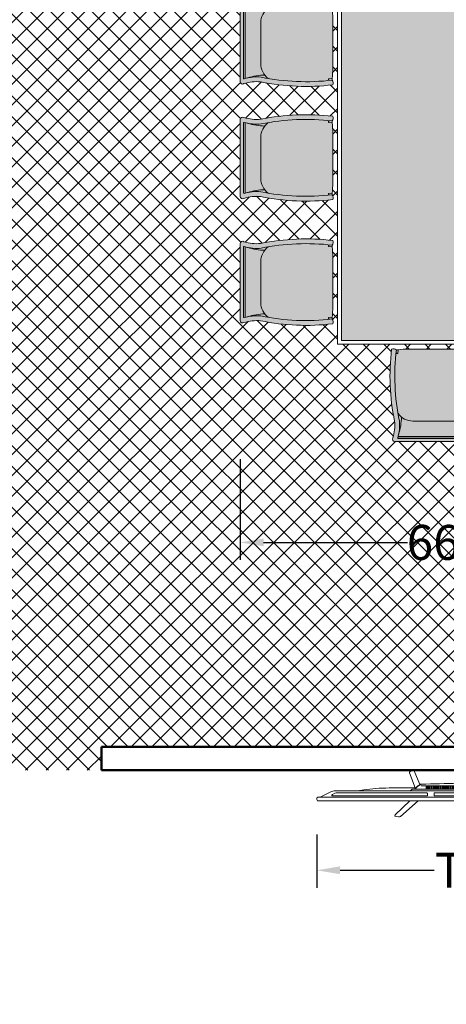
# Model space of a CAD drawing. Units: inches. Extents: x -466983 to 1020, y 324 to 318697.
# Tile 28 of 97: x 641 to 714, y 658 to 827. Entities that reach past the tile are written whole.
import ezdxf

# ---------------------------------------------------------------- set-up
doc = ezdxf.new("R2010")
doc.units = ezdxf.units.IN
doc.header["$MEASUREMENT"] = 0
for name, color, linetype, lineweight in [('A-ANNO-DIMS', 2, 'Continuous', 18), ('A-FLOR-PATT', 252, 'Continuous', 13), ('A-FURN', 8, 'Continuous', 18), ('A-WALL', 7, 'Continuous', 50)]:
    doc.layers.add(name, color=color, linetype=linetype, lineweight=lineweight)
doc.styles.get("Standard").update_dxf_attribs({"font": 'arial.ttf'})
doc.dimstyles.get("Standard").update_dxf_attribs({"dimtxt": 6, "dimasz": 4, "dimexe": 3, "dimexo": 3, "dimgap": 0.09, "dimtad": 0, "dimtih": 1, "dimtoh": 1, "dimdec": 1, "dimzin": 0, "dimdsep": 46, "dimlunit": 3, "dimtxsty": 'Standard', "dimcen": 0.09, "dimadec": 0, "dimazin": 0, "dimtfac": 1, "dimtdec": 1, "dimtofl": 0, "dimtmove": 0, "dimatfit": 3, "dimfxl": 1, "dimtolj": 1, "dimtzin": 0, "dimarcsym": 0})

# ---------------------------------------------------------------- blocks, each defined once
blk = doc.blocks.new('B2')
at = {"color": 0}
for points in [[(-161.1, -3.4), (-173.3, 26.2, 0.359324), (-175.3, 27.3, 0.097501), (-182.8, 24.2, 0.350578), (-183.5, 22.1), (-171.1, -10.4)], [(161.1, -3.4), (173.3, 26.2, -0.359324), (175.3, 27.3, -0.097501), (182.8, 24.2, -0.350578), (183.5, 22.1), (171.1, -10.4)], [(-381.9, -38.8, -0.13121), (-383.2, -32.7, -0.169032), (-383, -32.3), (-381.8, -31.1, -0.205713), (-381.3, -30.9), (-378.5, -30.9, 0.118206), (-376.2, -30.4), (-351.4, -18.4, -0.105648), (-345.8, -17), (0, -17)], [(-339.3, -21.2), (-339.3, -21.2, 0.099639), (-344.3, -22.2), (-349.2, -24.6, 0.215889), (-350.7, -26.3, 0.476075), (-349.4, -28, 0.244765)], [(-295.5, -17), (-282, -15, -0.02037), (-255.8, -12, -0.012056), (-227.2, -10.7), (-169.3, -10.7)], [(-181.8, -17), (-178.5, -14, -0.213415), (-177.3, -13.6), (0, -13.6)], [(-172.1, -13.6, -0.072098), (-159.2, -3, -0.121861), (-158.4, -2.8)], [(-170.1, -10.6, -0.053076), (-160.2, -2.9), (-158.4, -2.8)], [(-147.6, -13.6), (-147.6, -7.5, -0.414214), (-147.4, -7.3), (-146.5, -7.3, -0.414214), (-146.3, -7.5), (-146.3, -13.6)], [(-146.8, -28, 0.414214), (-145, -26.2), (-145, -23, 0.414214), (-146.8, -21.2)], [(-143.9, -13.6), (-143.9, -7.5, -0.414214), (-143.7, -7.3), (-142.7, -7.3, -0.414214), (-142.6, -7.5), (-142.6, -13.6)], [(-140.2, -13.6), (-140.2, -7.5, -0.414214), (-140, -7.3), (-139, -7.3, -0.414214), (-138.8, -7.5), (-138.8, -13.6)], [(-136.4, -13.6), (-136.4, -7.5, -0.414214), (-136.3, -7.3), (-135.3, -7.3, -0.414214), (-135.1, -7.5), (-135.1, -13.6)], [(-132.7, -13.6), (-132.7, -7.5, -0.414214), (-132.5, -7.3), (-131.6, -7.3, -0.414214), (-131.4, -7.5), (-131.4, -13.6)], [(-128.8, -28, -0.414214), (-130.6, -26.2), (-130.6, -23, -0.414214), (-128.8, -21.2)], [(-129, -13.6), (-129, -7.5, -0.414214), (-128.8, -7.3), (-127.9, -7.3, -0.414214), (-127.7, -7.5), (-127.7, -13.6)], [(-125.3, -13.6), (-125.3, -7.5, -0.414214), (-125.1, -7.3), (-124.1, -7.3, -0.414214), (-124, -7.5), (-124, -13.6)], [(-121.6, -13.6), (-121.6, -7.5, -0.414214), (-121.4, -7.3), (-120.4, -7.3, -0.414214), (-120.2, -7.5), (-120.2, -13.6)], [(-117.8, -13.6), (-117.8, -7.5, -0.414214), (-117.7, -7.3), (-116.7, -7.3, -0.414214), (-116.5, -7.5), (-116.5, -13.6)], [(-114.1, -13.6), (-114.1, -7.5, -0.414214), (-113.9, -7.3), (-113, -7.3, -0.414214), (-112.8, -7.5), (-112.8, -13.6)], [(-110.4, -13.6), (-110.4, -7.5, -0.414214), (-110.2, -7.3), (-109.3, -7.3, -0.414214), (-109.1, -7.5), (-109.1, -13.6)], [(-106.7, -13.6), (-106.7, -7.5, -0.414214), (-106.5, -7.3), (-105.5, -7.3, -0.414214), (-105.4, -7.5), (-105.4, -13.6)], [(-103, -13.6), (-103, -7.5, -0.414214), (-102.8, -7.3), (-101.8, -7.3, -0.414214), (-101.6, -7.5), (-101.6, -13.6)], [(-99.2, -13.6), (-99.2, -7.5, -0.414214), (-99.1, -7.3), (-98.1, -7.3, -0.414214), (-97.9, -7.5), (-97.9, -13.6)], [(-95.5, -13.6), (-95.5, -7.5, -0.414214), (-95.3, -7.3), (-94.4, -7.3, -0.414214), (-94.2, -7.5), (-94.2, -13.6)], [(-91.8, -13.6), (-91.8, -7.5, -0.414214), (-91.6, -7.3), (-90.7, -7.3, -0.414214), (-90.5, -7.5), (-90.5, -13.6)], [(-88.1, -13.6), (-88.1, -7.5, -0.414214), (-87.9, -7.3), (-86.9, -7.3, -0.414214), (-86.8, -7.5), (-86.8, -13.6)], [(-84.4, -13.6), (-84.4, -7.5, -0.414214), (-84.2, -7.3), (-83.2, -7.3, -0.414214), (-83, -7.5), (-83, -13.6)], [(-80.6, -13.6), (-80.6, -7.5, -0.414214), (-80.5, -7.3), (-79.5, -7.3, -0.414214), (-79.3, -7.5), (-79.3, -13.6)], [(-76.9, -13.6), (-76.9, -7.5, -0.414214), (-76.7, -7.3), (-75.8, -7.3, -0.414214), (-75.6, -7.5), (-75.6, -13.6)], [(-73.2, -13.6), (-73.2, -7.5, -0.414214), (-73, -7.3), (-72.1, -7.3, -0.414214), (-71.9, -7.5), (-71.9, -13.6)], [(-69.5, -13.6), (-69.5, -7.5, -0.414214), (-69.3, -7.3), (-68.3, -7.3, -0.414214), (-68.2, -7.5), (-68.2, -13.6)], [(-65.8, -13.6), (-65.8, -7.5, -0.414214), (-65.6, -7.3), (-64.6, -7.3, -0.414214), (-64.4, -7.5), (-64.4, -13.6)], [(-62, -13.6), (-62, -7.5, -0.414214), (-61.9, -7.3), (-60.9, -7.3, -0.414214), (-60.7, -7.5), (-60.7, -13.6)], [(-58.3, -13.6), (-58.3, -7.5, -0.414214), (-58.1, -7.3), (-57.2, -7.3, -0.414214), (-57, -7.5), (-57, -13.6)], [(-54.6, -13.6), (-54.6, -7.5, -0.414214), (-54.4, -7.3), (-53.5, -7.3, -0.414214), (-53.3, -7.5), (-53.3, -13.6)], [(-50.9, -13.6), (-50.9, -7.5, -0.414214), (-50.7, -7.3), (-49.7, -7.3, -0.414214), (-49.6, -7.5), (-49.6, -13.6)], [(-47.2, -13.6), (-47.2, -7.5, -0.414214), (-47, -7.3), (-46, -7.3, -0.414214), (-45.8, -7.5), (-45.8, -13.6)], [(-43.4, -13.6), (-43.4, -7.5, -0.414214), (-43.3, -7.3), (-42.3, -7.3, -0.414214), (-42.1, -7.5), (-42.1, -13.6)], [(-39.7, -13.6), (-39.7, -7.5, -0.414214), (-39.5, -7.3), (-38.6, -7.3, -0.414214), (-38.4, -7.5), (-38.4, -13.6)], [(-36, -13.6), (-36, -7.5, -0.414214), (-35.8, -7.3), (-34.9, -7.3, -0.414214), (-34.7, -7.5), (-34.7, -13.6)], [(-32.3, -13.6), (-32.3, -7.5, -0.414214), (-32.1, -7.3), (-31.1, -7.3, -0.414214), (-31, -7.5), (-31, -13.6)], [(-28.6, -13.6), (-28.6, -7.5, -0.414214), (-28.4, -7.3), (-27.4, -7.3, -0.414214), (-27.2, -7.5), (-27.2, -13.6)], [(-24.8, -13.6), (-24.8, -7.5, -0.414214), (-24.7, -7.3), (-23.7, -7.3, -0.414214), (-23.5, -7.5), (-23.5, -13.6)], [(-21.1, -13.6), (-21.1, -7.5, -0.414214), (-20.9, -7.3), (-20, -7.3, -0.414214), (-19.8, -7.5), (-19.8, -13.6)], [(-17.4, -13.6), (-17.4, -7.5, -0.414214), (-17.2, -7.3), (-16.3, -7.3, -0.414214), (-16.1, -7.5), (-16.1, -13.6)], [(-13.7, -13.6), (-13.7, -7.5, -0.414214), (-13.5, -7.3), (-12.5, -7.3, -0.414214), (-12.4, -7.5), (-12.4, -13.6)], [(-10, -13.6), (-10, -7.5, -0.414214), (-9.8, -7.3), (-8.8, -7.3, -0.414214), (-8.6, -7.5), (-8.6, -13.6)], [(-10, -28, 0.414214), (-8.2, -26.2), (-8.2, -23, 0.414214), (-10, -21.2)], [(-6.2, -13.6), (-6.2, -7.5, -0.414214), (-6.1, -7.3), (-5.1, -7.3, -0.414214), (-4.9, -7.5), (-4.9, -13.6)], [(-2.5, -13.6), (-2.5, -7.5, -0.414214), (-2.3, -7.3), (-1.4, -7.3, -0.414214), (-1.2, -7.5), (-1.2, -13.6)], [(181.8, -17), (178.5, -14, 0.213415), (177.3, -13.6), (0, -13.6)], [(381.9, -38.8, 0.13121), (383.2, -32.7, 0.169032), (383, -32.3), (381.8, -31.1, 0.205713), (381.3, -30.9), (378.5, -30.9, -0.118206), (376.2, -30.4), (351.4, -18.4, 0.105648), (345.8, -17), (0, -17)], [(2.5, -13.6), (2.5, -7.5, 0.414214), (2.3, -7.3), (1.4, -7.3, 0.414214), (1.2, -7.5), (1.2, -13.6)], [(6.2, -13.6), (6.2, -7.5, 0.414214), (6.1, -7.3), (5.1, -7.3, 0.414214), (4.9, -7.5), (4.9, -13.6)], [(10, -28, -0.414214), (8.2, -26.2), (8.2, -23, -0.414214), (10, -21.2)], [(10, -13.6), (10, -7.5, 0.414214), (9.8, -7.3), (8.8, -7.3, 0.414214), (8.6, -7.5), (8.6, -13.6)], [(13.7, -13.6), (13.7, -7.5, 0.414214), (13.5, -7.3), (12.5, -7.3, 0.414214), (12.4, -7.5), (12.4, -13.6)], [(17.4, -13.6), (17.4, -7.5, 0.414214), (17.2, -7.3), (16.3, -7.3, 0.414214), (16.1, -7.5), (16.1, -13.6)], [(21.1, -13.6), (21.1, -7.5, 0.414214), (20.9, -7.3), (20, -7.3, 0.414214), (19.8, -7.5), (19.8, -13.6)], [(24.8, -13.6), (24.8, -7.5, 0.414214), (24.7, -7.3), (23.7, -7.3, 0.414214), (23.5, -7.5), (23.5, -13.6)], [(28.6, -13.6), (28.6, -7.5, 0.414214), (28.4, -7.3), (27.4, -7.3, 0.414214), (27.2, -7.5), (27.2, -13.6)], [(32.3, -13.6), (32.3, -7.5, 0.414214), (32.1, -7.3), (31.1, -7.3, 0.414214), (31, -7.5), (31, -13.6)], [(36, -13.6), (36, -7.5, 0.414214), (35.8, -7.3), (34.9, -7.3, 0.414214), (34.7, -7.5), (34.7, -13.6)], [(39.7, -13.6), (39.7, -7.5, 0.414214), (39.5, -7.3), (38.6, -7.3, 0.414214), (38.4, -7.5), (38.4, -13.6)], [(43.4, -13.6), (43.4, -7.5, 0.414214), (43.3, -7.3), (42.3, -7.3, 0.414214), (42.1, -7.5), (42.1, -13.6)], [(47.2, -13.6), (47.2, -7.5, 0.414214), (47, -7.3), (46, -7.3, 0.414214), (45.8, -7.5), (45.8, -13.6)], [(50.9, -13.6), (50.9, -7.5, 0.414214), (50.7, -7.3), (49.7, -7.3, 0.414214), (49.6, -7.5), (49.6, -13.6)], [(54.6, -13.6), (54.6, -7.5, 0.414214), (54.4, -7.3), (53.5, -7.3, 0.414214), (53.3, -7.5), (53.3, -13.6)], [(58.3, -13.6), (58.3, -7.5, 0.414214), (58.1, -7.3), (57.2, -7.3, 0.414214), (57, -7.5), (57, -13.6)], [(62, -13.6), (62, -7.5, 0.414214), (61.9, -7.3), (60.9, -7.3, 0.414214), (60.7, -7.5), (60.7, -13.6)], [(65.8, -13.6), (65.8, -7.5, 0.414214), (65.6, -7.3), (64.6, -7.3, 0.414214), (64.4, -7.5), (64.4, -13.6)], [(69.5, -13.6), (69.5, -7.5, 0.414214), (69.3, -7.3), (68.3, -7.3, 0.414214), (68.2, -7.5), (68.2, -13.6)], [(73.2, -13.6), (73.2, -7.5, 0.414214), (73, -7.3), (72.1, -7.3, 0.414214), (71.9, -7.5), (71.9, -13.6)], [(76.9, -13.6), (76.9, -7.5, 0.414214), (76.7, -7.3), (75.8, -7.3, 0.414214), (75.6, -7.5), (75.6, -13.6)], [(80.6, -13.6), (80.6, -7.5, 0.414214), (80.5, -7.3), (79.5, -7.3, 0.414214), (79.3, -7.5), (79.3, -13.6)], [(84.4, -13.6), (84.4, -7.5, 0.414214), (84.2, -7.3), (83.2, -7.3, 0.414214), (83, -7.5), (83, -13.6)], [(88.1, -13.6), (88.1, -7.5, 0.414214), (87.9, -7.3), (86.9, -7.3, 0.414214), (86.8, -7.5), (86.8, -13.6)], [(91.8, -13.6), (91.8, -7.5, 0.414214), (91.6, -7.3), (90.7, -7.3, 0.414214), (90.5, -7.5), (90.5, -13.6)], [(95.5, -13.6), (95.5, -7.5, 0.414214), (95.3, -7.3), (94.4, -7.3, 0.414214), (94.2, -7.5), (94.2, -13.6)], [(99.2, -13.6), (99.2, -7.5, 0.414214), (99.1, -7.3), (98.1, -7.3, 0.414214), (97.9, -7.5), (97.9, -13.6)], [(103, -13.6), (103, -7.5, 0.414214), (102.8, -7.3), (101.8, -7.3, 0.414214), (101.6, -7.5), (101.6, -13.6)], [(106.7, -13.6), (106.7, -7.5, 0.414214), (106.5, -7.3), (105.5, -7.3, 0.414214), (105.4, -7.5), (105.4, -13.6)], [(110.4, -13.6), (110.4, -7.5, 0.414214), (110.2, -7.3), (109.3, -7.3, 0.414214), (109.1, -7.5), (109.1, -13.6)], [(114.1, -13.6), (114.1, -7.5, 0.414214), (113.9, -7.3), (113, -7.3, 0.414214), (112.8, -7.5), (112.8, -13.6)], [(117.8, -13.6), (117.8, -7.5, 0.414214), (117.7, -7.3), (116.7, -7.3, 0.414214), (116.5, -7.5), (116.5, -13.6)], [(121.6, -13.6), (121.6, -7.5, 0.414214), (121.4, -7.3), (120.4, -7.3, 0.414214), (120.2, -7.5), (120.2, -13.6)], [(125.3, -13.6), (125.3, -7.5, 0.414214), (125.1, -7.3), (124.1, -7.3, 0.414214), (124, -7.5), (124, -13.6)], [(129, -13.6), (129, -7.5, 0.414214), (128.8, -7.3), (127.9, -7.3, 0.414214), (127.7, -7.5), (127.7, -13.6)], [(128.8, -28, 0.414214), (130.6, -26.2), (130.6, -23, 0.414214), (128.8, -21.2)], [(132.7, -13.6), (132.7, -7.5, 0.414214), (132.5, -7.3), (131.6, -7.3, 0.414214), (131.4, -7.5), (131.4, -13.6)], [(136.4, -13.6), (136.4, -7.5, 0.414214), (136.3, -7.3), (135.3, -7.3, 0.414214), (135.1, -7.5), (135.1, -13.6)], [(140.2, -13.6), (140.2, -7.5, 0.414214), (140, -7.3), (139, -7.3, 0.414214), (138.8, -7.5), (138.8, -13.6)], [(143.9, -13.6), (143.9, -7.5, 0.414214), (143.7, -7.3), (142.7, -7.3, 0.414214), (142.6, -7.5), (142.6, -13.6)], [(146.8, -28, -0.414214), (145, -26.2), (145, -23, -0.414214), (146.8, -21.2)], [(147.6, -13.6), (147.6, -7.5, 0.414214), (147.4, -7.3), (146.5, -7.3, 0.414214), (146.3, -7.5), (146.3, -13.6)], [(172.1, -13.6, 0.072098), (159.2, -3, 0.121861), (158.4, -2.8)], [(170.1, -10.6, 0.053076), (160.2, -2.9), (158.4, -2.8)], [(295.5, -17), (282, -15, 0.02037), (255.8, -12, 0.012056), (227.2, -10.7), (169.3, -10.7)], [(339.3, -21.2), (339.3, -21.2, -0.099639), (344.3, -22.2), (349.2, -24.6, -0.215889), (350.7, -26.3, -0.476075), (349.4, -28, -0.244765)], [(-182.5, -38.8), (-214.4, -69.1, 0.250582), (-215, -71, 0.266718), (-214.3, -71.9, 0.084688)], [(-214.3, -71.9), (-207.3, -73.1, 0.211205), (-203.3, -72.1), (-165.2, -38.8)], [(214.3, -71.9), (207.3, -73.1, -0.211205), (203.3, -72.1), (165.2, -38.8)], [(182.5, -38.8), (214.4, -69.1, -0.250582), (215, -71, -0.266718), (214.3, -71.9, -0.084688)]]:
    blk.add_lwpolyline(points, format="xyb", dxfattribs=at)
for points in [[(-339.3, -21.2), (-146.8, -21.2)], [(-158.6, -6.5), (0, -6.5)], [(-128.8, -21.2), (-10, -21.2)], [(158.6, -6.5), (0, -6.5)], [(128.8, -21.2), (10, -21.2)], [(339.3, -21.2), (146.8, -21.2)], [(-381.9, -38.8), (0, -38.8)], [(-378.5, -30.9), (0, -30.9)], [(-349.4, -28), (-146.8, -28)], [(-128.8, -28), (-10, -28)], [(378.5, -30.9), (0, -30.9)], [(381.9, -38.8), (0, -38.8)], [(128.8, -28), (10, -28)], [(349.4, -28), (146.8, -28)]]:
    blk.add_lwpolyline(points, dxfattribs=at)
for centre, radius, start, end in [((0, -4564), 4564, 90, 91.9893), ((0, -4564), 4564, 88.0107, 90), ((-170.5, -10.1), 0.6, 200.9784, 314.0295), ((170.5, -10.1), 0.6, 225.9705, 339.0216)]:
    blk.add_arc(centre, radius, start, end, dxfattribs=at)
blk = doc.blocks.new('A$C51F1')
h = blk.add_hatch(color=256)
h.dxf.hatch_style = 1
h.paths.add_polyline_path([(0.4279, 0.4929), (0.026, 0.4929, 0.585109), (0.0153, 0.4737, -0.102523), (0.0249, 0.3863, 0.080461), (0.0093, 0.0091, 0.3023), (0.0338, 0.012, -0.012942), (0.0343, 0.0123, -0.080591), (0.05, 0.3835, 0.086627), (0.0435, 0.4661, -0.308377), (0.0433, 0.4665, -0.237278), (0.0433, 0.4671, 0.005839), (0.0418, 0.4726, -0.471786), (0.0436, 0.4758), (0.2273, 0.4758), (0.4111, 0.4758, -0.471786), (0.4129, 0.4726, 0.005839), (0.4114, 0.4671, -0.293853), (0.4112, 0.4664, 0.08699), (0.4047, 0.3835, -0.080655), (0.4203, 0.012, 0.301773), (0.4447, 0.0091, 0.080461), (0.4291, 0.3863, -0.102523), (0.4387, 0.4737, 0.587111)])
h.paths.add_polyline_path([(0.4107, 0.4676), (0.2273, 0.4676), (0.0439, 0.4676, 0.311255), (0.0433, 0.4671, -0.000568), (0.0434, 0.4666, -0.365297), (0.0439, 0.4668), (0.2273, 0.4668), (0.4107, 0.4668, -0.365297), (0.4113, 0.4666, -0.000568), (0.4114, 0.4671, 0.311255)], flags=17)
h = blk.add_hatch(color=256)
h.dxf.hatch_style = 1
h.paths.add_polyline_path([(0.4117, 0.3464, 0.23459), (0.3341, 0.3858), (0.2273, 0.3858), (0.1205, 0.3858, 0.165743), (0.061, 0.3649, 0.071703), (0.0463, 0.4542, -0.071168), (0.0502, 0.3861, 0.080361), (0.0343, 0.0123, -0.184513), (0.0429, 0.0127, 0.028193), (0.097, 0.0091), (0.227, 0.0091), (0.3571, 0.0091, 0.028193), (0.4111, 0.0127, -0.198751), (0.4203, 0.012, 0.072468)])
h.paths.add_polyline_path([(0.4084, 0.4542, -0.01323), (0.4113, 0.4666, 0.365297), (0.4107, 0.4668, 0.310553), (0.4107, 0.4676), (0.0439, 0.4676, 0.311255), (0.0433, 0.4671, -0.013798), (0.0463, 0.4542, -0.071703), (0.061, 0.3649, -0.165743), (0.1205, 0.3858), (0.2273, 0.3858), (0.3341, 0.3858, -0.165743), (0.3937, 0.3649, -0.071703)])
h.paths.add_polyline_path([(0.4047, 0.3835, -0.073923), (0.4084, 0.4542, 0.071703), (0.3937, 0.3649, -0.06627), (0.4117, 0.3464, 0.008137)], flags=17)
h.paths.add_polyline_path([(0.413, 0.473, 0.415817), (0.4111, 0.4758), (0.0436, 0.4758, 0.415817), (0.0416, 0.473, -0.006308), (0.0433, 0.4671, -0.311255), (0.0439, 0.4676), (0.4107, 0.4676, -0.336555), (0.4114, 0.4671, -0.006308)])
h = blk.add_hatch(color=256)
h.dxf.hatch_style = 1
h.paths.add_polyline_path([(0.4084, 0.4542, -0.01323), (0.4113, 0.4666, 0.365297), (0.4107, 0.4668), (0.2273, 0.4668), (0.0436, 0.4668, 0.193526), (0.0434, 0.4666, -0.01323), (0.0463, 0.4542, -0.071703), (0.061, 0.3649, -0.165743), (0.1205, 0.3858), (0.2273, 0.3858), (0.3341, 0.3858, -0.165743), (0.3937, 0.3649, -0.071703)])
at = {"color": 0}
for p, q in [((0.0436, 0.4758), (0.4111, 0.4758)), ((0.0439, 0.4676), (0.4107, 0.4676)), ((0.2273, 0.4668), (0.0439, 0.4668)), ((0.2273, 0.4668), (0.4107, 0.4668)), ((0.2273, 0.3858), (0.1205, 0.3858)), ((0.2273, 0.3858), (0.3341, 0.3858)), ((0.0417, 0.0321), (0.0321, 0.0321)), ((0.0417, 0.0321), (0.0326, 0.0278)), ((0.0435, 0.0127), (0.0417, 0.0321)), ((0.4112, 0.0127), (0.4129, 0.0321)), ((0.4129, 0.0321), (0.4225, 0.0321)), ((0.4129, 0.0321), (0.4221, 0.0278))]:
    blk.add_line(p, q, dxfattribs=at)
blk.add_lwpolyline([(0.4387, 0.4737, 0.102523), (0.4291, 0.3863, -0.080461), (0.4447, 0.0091, -0.3023), (0.4203, 0.012, 0.197932), (0.4111, 0.0127, -0.028193), (0.3571, 0.0091), (0.227, 0.0091), (0.097, 0.0091, -0.028193), (0.0429, 0.0127, 0.197932), (0.0338, 0.012, -0.3023), (0.0093, 0.0091, -0.080461), (0.0249, 0.3863, 0.102523), (0.0153, 0.4737, -0.587111), (0.0261, 0.4929), (0.4279, 0.4929, -0.587111)], format="xyb", close=True, dxfattribs=at)
for centre, radius, start, end in [((0.044, 0.4735), 0.00242, 100.345, 201.3742), ((-0.1898, 0.4063), 0.2409, 355.1793, 16.07), ((0.0439, 0.4669), 0.000725, 87.3762, 197.5208), ((0.0438, 0.4664), 0.000433, 71.7715, 189.2202), ((0.6445, 0.4063), 0.2409, 164.0374, 185.4487), ((0.4107, 0.4669), 0.000725, 342.4792, 92.6238), ((0.4109, 0.4664), 0.000433, 350.7798, 108.2285), ((0.4106, 0.4735), 0.00242, 338.6258, 79.655), ((-0.2563, 0.3584), 0.3173, 1.1591, 17.5641), ((0.7109, 0.3584), 0.3173, 162.4359, 178.8409), ((1.1976, 0.1501), 1.1714, 168.378, 186.769), ((0.1214, 0.2879), 0.0978, 90.5164, 143.1927), ((0.3332, 0.2879), 0.0978, 36.8073, 89.4836), ((-0.7314, 0.1497), 1.1599, 353.1854, 11.6291), ((0.0397, 0.0013), 0.012, 71.7536, 116.5375), ((0.4149, 0.0013), 0.012, 63.4625, 108.2464)]:
    blk.add_arc(centre, radius, start, end, dxfattribs=at)
blk = doc.blocks.new('Dining Table 1')
h = blk.add_hatch(color=256)
h.dxf.hatch_style = 1
h.set_gradient(color1=(0, 107, 0), color2=(254, 234, 185), name='INVSPHERICAL')
h.paths.add_polyline_path([(1939.98, 1142.68), (1908.44, 1142.68), (1908.44, 1061.84), (1939.98, 1061.84)])
at = {"ltscale": 0.5}
for points in [[(1907.78, 1143.33), (1907.78, 1061.19), (1940.64, 1061.19), (1940.64, 1143.33)], [(1908.44, 1142.68), (1908.44, 1061.84), (1939.98, 1061.84), (1939.98, 1142.68)]]:
    blk.add_lwpolyline(points, close=True, dxfattribs=at)
at = {"ltscale": 0.5, "xscale": 32.85880592291654, "yscale": 32.85880592291654, "zscale": 32.85880592291654}
blk.add_blockref('A$C51F1', (1916.75, 1143.86), dxfattribs=at)
at = {"ltscale": 0.5, "yscale": 32.85880592291654, "zscale": 32.85880592291654}
for p, xscale, rotation in [((1907.26, 1140.11), -32.85880592291654, 90), ((1941.16, 1140.11), 32.85880592291654, 270), ((1907.26, 1120.4), -32.85880592291654, 90), ((1941.16, 1120.4), 32.85880592291654, 270), ((1907.26, 1085.76), 32.85880592291654, 89.99999999999999), ((1941.16, 1085.76), -32.85880592291654, 270), ((1907.26, 1064.41), 32.85880592291654, 89.99999999999999), ((1941.16, 1064.41), -32.85880592291654, 270), ((1916.75, 1060.66), -32.85880592291654, 180)]:
    blk.add_blockref('A$C51F1', p, dxfattribs=dict(at, xscale=xscale, rotation=rotation))
blk = doc.blocks.new('*D101')
at = {"layer": 'A-ANNO-DIMS', "color": 0, "lineweight": -2, "transparency": 16777216}
for p, q in [((691.81, 686.91), (691.81, 677.75)), ((752.9, 686.91), (752.9, 677.75)), ((695.81, 680.75), (711.95, 680.75)), ((748.9, 680.75), (732.76, 680.75))]:
    blk.add_line(p, q, dxfattribs=at)
at = {"layer": 'A-ANNO-DIMS', "color": 0, "transparency": 16777216}
for points in [[(695.81, 681.42), (695.81, 680.08), (691.81, 680.75)], [(748.9, 681.42), (748.9, 680.08), (752.9, 680.75)]]:
    blk.add_solid(points, dxfattribs=at)
at = {"layer": 'Defpoints', "color": 0, "transparency": 16777216}
for p in [(691.81, 689.91), (752.9, 689.91), (752.9, 680.75)]:
    blk.add_point(p, dxfattribs=at)
at = {"layer": 'A-ANNO-DIMS', "color": 0, "transparency": 16777216, "insert": (722.35, 680.75), "char_height": 6, "attachment_point": 5}
blk.add_mtext('\\A1;TV 61', dxfattribs=at)
blk = doc.blocks.new('*D112')
at = {"layer": 'A-ANNO-DIMS', "color": 0, "lineweight": -2, "transparency": 16777216}
for p, q in [((678.65, 751.43), (678.65, 734.1)), ((744.94, 751.43), (744.94, 734.1)), ((682.65, 737.1), (707.39, 737.1)), ((740.94, 737.1), (716.2, 737.1))]:
    blk.add_line(p, q, dxfattribs=at)
at = {"layer": 'A-ANNO-DIMS', "color": 0, "transparency": 16777216}
for points in [[(682.65, 737.76), (682.65, 736.43), (678.65, 737.1)], [(740.94, 737.76), (740.94, 736.43), (744.94, 737.1)]]:
    blk.add_solid(points, dxfattribs=at)
at = {"layer": 'Defpoints', "color": 0, "transparency": 16777216}
for p in [(678.65, 754.43), (744.94, 754.43), (744.94, 737.1)]:
    blk.add_point(p, dxfattribs=at)
at = {"layer": 'A-ANNO-DIMS', "color": 0, "transparency": 16777216, "insert": (711.79, 737.1), "char_height": 6, "attachment_point": 5}
blk.add_mtext('\\A1;66', dxfattribs=at)

msp = doc.modelspace()

# ---------------------------------------------------------------- hatches: boundary and pattern name
at = {"layer": 'A-FLOR-PATT', "transparency": 33554572}
h = msp.add_hatch(dxfattribs=at)
h.set_pattern_fill('ANSI37', color=256, scale=30)
h.set_pattern_definition([(45, (-1212.4137, -290.035), (-2.6516504, 2.6516504), []), (135, (-1212.4137, -290.035), (-2.6516504, -2.6516504), [])])
h.paths.add_polyline_path([(901.81, 1075.94), (900.61, 1075.94), (900.61, 1065.39), (899.39, 1065.39), (898.09, 1065.39), (892.84, 1058.71, -0.258377), (892.19, 1058.35), (879.98, 1058.35, -0.20177), (879.44, 1058.58), (874.08, 1065.39), (872.78, 1065.39), (871.56, 1065.39), (871.56, 1075.94), (813.81, 1075.94), (813.81, 1044.79), (832.39, 1044.79, -0.394795), (848.66, 1028.54), (848.66, 1009.94), (901.81, 1009.94), (901.81, 1015.94), (901.31, 1015.94), (871.31, 1015.94), (871.31, 1017.25), (871.33, 1017.25, -0.401453), (901.31, 1045.94), (901.81, 1045.94)])
edge = h.paths.add_edge_path(flags=16)
edge.add_line((847.77, 1068.95), (847.77, 1073.71))
edge.add_arc((849.23, 1073.71), 1.45, 90, 180, ccw=False)
edge.add_line((849.23, 1075.16), (864.49, 1075.16))
edge.add_arc((864.49, 1073.71), 1.45, 0, 90, ccw=False)
edge.add_line((865.95, 1073.71), (865.95, 1069))
edge.add_arc((832.64, 1068.98), 33.3, -20.6123, 0.0472, ccw=False)
edge.add_ellipse((856.86, 1058.48), major_axis=(0, 10.21), ratio=0.685919, start_angle=100.0088, end_angle=259.9912, ccw=False)
edge.add_arc((881.07, 1068.98), 33.3, 180.0472, 200.6123, ccw=False)
h.paths.add_polyline_path([(853.15, 1066.48), (853.15, 1066.45), (853.15, 1066.45, 0.433107), (852.92, 1066.68), (852.92, 1066.45), (853.15, 1066.45), (853.15, 1066.48), (853.09, 1066.61, 0.697939), (852.7, 1066.45), (852.7, 1066.45), (852.7, 1066.48), (852.92, 1067), (852.92, 1066.68, -0.396254)], flags=0)
h.paths.add_polyline_path([(861.02, 1066.48), (861.02, 1066.45), (861.02, 1066.45, 0.416404), (860.8, 1066.68), (860.8, 1066.45), (861.02, 1066.45), (861.02, 1066.48), (860.97, 1066.61, 0.713344), (860.57, 1066.45), (860.57, 1066.45), (860.57, 1066.48), (860.8, 1067), (860.8, 1066.68, -0.379973)], flags=0)
edge = h.paths.add_edge_path(flags=0)
edge.add_spline(control_points=[(861.13, 1065.79), (861.47, 1065.25), (861.61, 1065.02), (861.98, 1064.37), (862.19, 1063.94), (862.56, 1063.04), (862.72, 1062.56), (862.99, 1061.58), (863.09, 1061.07), (863.25, 1060.03), (863.29, 1059.5), (863.33, 1058.44), (863.32, 1057.91), (863.24, 1056.85), (863.17, 1056.33), (862.97, 1055.31), (862.84, 1054.81), (862.54, 1053.85), (862.36, 1053.39), (861.95, 1052.52), (861.73, 1052.12), (861.23, 1051.36), (860.97, 1051.02), (860.4, 1050.39), (860.11, 1050.12), (859.49, 1049.65), (859.18, 1049.45), (858.53, 1049.13), (858.2, 1049.01), (857.53, 1048.85), (857.2, 1048.81), (856.52, 1048.81), (856.19, 1048.85), (855.52, 1049.01), (855.19, 1049.13), (854.54, 1049.45), (854.23, 1049.64), (853.61, 1050.12), (853.32, 1050.39), (852.75, 1051.01), (852.49, 1051.36), (852, 1052.11), (851.77, 1052.52), (851.36, 1053.39), (851.18, 1053.85), (850.88, 1054.81), (850.75, 1055.31), (850.55, 1056.33), (850.48, 1056.85), (850.4, 1057.9), (850.39, 1058.44), (850.43, 1059.5), (850.47, 1060.03), (850.63, 1061.07), (850.73, 1061.58), (851, 1062.56), (851.16, 1063.04), (851.53, 1063.94), (851.73, 1064.37), (852.11, 1065.02), (852.25, 1065.25), (852.61, 1065.73)], knot_values=[3.915332, 3.915332, 3.915332, 3.915332, 4.013468, 4.013468, 4.175532, 4.175532, 4.337596, 4.337596, 4.49966, 4.49966, 4.661724, 4.661724, 4.823788, 4.823788, 4.985852, 4.985852, 5.147916, 5.147916, 5.30998, 5.30998, 5.472044, 5.472044, 5.634109, 5.634109, 5.796173, 5.796173, 5.958237, 5.958237, 6.120301, 6.120301, 6.282365, 6.282365, 6.444429, 6.444429, 6.606493, 6.606493, 6.768557, 6.768557, 6.930621, 6.930621, 7.092685, 7.092685, 7.254749, 7.254749, 7.416813, 7.416813, 7.578878, 7.578878, 7.740942, 7.740942, 7.903006, 7.903006, 8.06507, 8.06507, 8.227134, 8.227134, 8.389198, 8.389198, 8.551262, 8.551262, 8.65037, 8.65037, 8.65037, 8.65037], degree=3, periodic=0)
edge.add_line((852.64, 1065.79), (861.13, 1065.79))
edge = h.paths.add_edge_path(flags=0)
edge.add_ellipse((856.85, 1057.74), major_axis=(0, 7.79), ratio=0.687861, start_angle=0, end_angle=360)
h.paths.add_polyline_path([(848.86, 1069.39), (848.86, 1073.96, -0.414214), (849.95, 1075.05), (863.77, 1075.05, -0.414214), (864.86, 1073.96), (864.86, 1069.39, -0.388936), (864.52, 1069.03, -0.043561), (849.2, 1069.03, -0.388936)], flags=0)
h.paths.add_polyline_path([(853.1, 1068.11, -1), (852.68, 1068.11, -1)], flags=0)
edge = h.paths.add_edge_path(flags=0)
edge.add_ellipse((856.86, 1057.34), major_axis=(0, 2.21), ratio=0.657164, start_angle=0, end_angle=360)
h.paths.add_polyline_path([(861.04, 1068.11, -1), (860.62, 1068.11, -1)], flags=0)
edge = h.paths.add_edge_path()
edge.add_line((573.95, 1057.34), (573.95, 1075.94))
edge.add_line((573.95, 1075.94), (558.73, 1075.94))
edge.add_line((558.73, 1075.94), (558.73, 1065.39))
edge.add_line((558.73, 1065.39), (557.51, 1065.39))
edge.add_line((557.51, 1065.39), (556.21, 1065.39))
edge.add_line((556.21, 1065.39), (550.95, 1058.71))
edge.add_arc((550.3, 1059.12), 0.765, 270, 327.9483, ccw=False)
edge.add_line((550.3, 1058.35), (538.1, 1058.35))
edge.add_arc((538.1, 1059.12), 0.765, 224.3704, 270, ccw=False)
edge.add_line((537.55, 1058.58), (532.2, 1065.39))
edge.add_line((532.2, 1065.39), (530.9, 1065.39))
edge.add_line((530.9, 1065.39), (529.67, 1065.39))
edge.add_line((529.67, 1065.39), (529.67, 1075.94))
edge.add_line((529.67, 1075.94), (520.81, 1075.94))
edge.add_line((520.81, 1075.94), (520.81, 1045.94))
edge.add_line((520.81, 1045.94), (521.31, 1045.94))
edge.add_arc((521.31, 1015.94), 30, 2.5075, 90, ccw=False)
edge.add_line((551.28, 1017.25), (551.31, 1017.25))
edge.add_line((551.31, 1017.25), (551.31, 1015.94))
edge.add_line((551.31, 1015.94), (520.81, 1015.94))
edge.add_line((520.81, 1015.94), (520.81, 1009.94))
edge.add_line((520.81, 1009.94), (559.19, 1010.4))
edge.add_arc((559.19, 1011.86), 1.45, 180, 270, ccw=False)
edge.add_line((557.74, 1011.86), (557.74, 1016.56))
edge.add_arc((591.04, 1016.59), 33.3, 159.3877, 180.0472, ccw=False)
edge.add_ellipse((566.82, 1027.08), major_axis=(0, 10.21), ratio=0.685919, start_angle=280.0088, end_angle=439.9912, ccw=False)
edge.add_arc((542.61, 1016.59), 33.3, 0.0472, 20.6123, ccw=False)
edge.add_line((575.91, 1016.62), (575.91, 1011.86))
edge.add_arc((574.46, 1011.86), 1.45, -90, 0, ccw=False)
edge.add_line((574.46, 1010.4), (608.81, 1009.94))
edge.add_line((608.81, 1009.94), (608.81, 1041.09))
edge.add_line((608.81, 1041.09), (590.22, 1041.09))
edge.add_arc((590.78, 1057.91), 16.83, 181.9277, 268.1032, ccw=False)
edge = h.paths.add_edge_path()
edge.add_ellipse((494.24, 583.62), major_axis=(0, 10.21), ratio=0.685919, start_angle=280.0088, end_angle=439.9912, ccw=False)
edge.add_arc((470.03, 573.12), 33.3, 0.0472, 20.6123, ccw=False)
edge.add_line((503.33, 573.15), (503.33, 568.39))
edge.add_arc((501.88, 568.39), 1.45, -90, 0, ccw=False)
edge.add_line((501.88, 566.94), (539.81, 566.94))
edge.add_line((539.81, 566.94), (539.81, 572.94))
edge.add_line((539.81, 572.94), (539.31, 572.94))
edge.add_line((539.31, 572.94), (509.31, 572.94))
edge.add_line((509.31, 572.94), (509.31, 574.25))
edge.add_line((509.31, 574.25), (509.33, 574.25))
edge.add_arc((539.31, 572.94), 30, 90, 177.4925, ccw=False)
edge.add_line((539.31, 602.94), (539.81, 602.94))
edge.add_line((539.81, 602.94), (539.81, 626.94))
edge.add_line((539.81, 626.94), (531.77, 626.94))
edge.add_line((531.77, 626.94), (531.77, 616.39))
edge.add_line((531.77, 616.39), (530.55, 616.39))
edge.add_line((530.55, 616.39), (529.25, 616.39))
edge.add_line((529.25, 616.39), (523.71, 609.35))
edge.add_line((523.71, 609.35), (510.78, 609.35))
edge.add_line((510.78, 609.35), (505.24, 616.39))
edge.add_line((505.24, 616.39), (503.94, 616.39))
edge.add_line((503.94, 616.39), (502.72, 616.39))
edge.add_line((502.72, 616.39), (502.72, 626.94))
edge.add_line((502.72, 626.94), (481.7, 626.94))
edge.add_line((481.7, 626.94), (481.7, 611))
edge.add_arc((467.27, 611.47), 14.44, 271.9277, 358.1032, ccw=False)
edge.add_line((467.76, 597.05), (451.81, 597.05))
edge.add_line((451.81, 597.05), (451.81, 584.4))
edge.add_line((451.81, 584.4), (451.81, 566.94))
edge.add_line((451.81, 566.94), (486.61, 566.94))
edge.add_arc((486.61, 568.39), 1.45, 180, 270, ccw=False)
edge.add_line((485.16, 568.39), (485.16, 573.1))
edge.add_arc((518.46, 573.12), 33.3, 159.3877, 180.0472, ccw=False)
h.paths.add_polyline_path([(836.26, 1020.73), (879.89, 1020.73), (879.89, 1039.39), (836.26, 1039.39)], flags=25)
h.paths.add_polyline_path([(549.99, 1036.75), (593.61, 1036.75), (593.61, 1055.41), (549.99, 1055.41)], flags=24)
h.paths.add_polyline_path([(475.12, 595.6), (518.75, 595.6), (518.75, 614.25), (475.12, 614.25)], flags=24)
h = msp.add_hatch(dxfattribs=at)
h.set_pattern_fill('ANSI37', color=256, scale=20)
h.set_pattern_definition([(45, (-1212.4137, -290.035), (-1.767767, 1.767767), []), (135, (-1212.4137, -290.035), (-1.767767, -1.767767), [])])
h.paths.add_polyline_path([(809.81, 870.94), (809.81, 888.15), (807, 888.15), (802.66, 888.15), (789.38, 888.15), (786.28, 888.15, -0.414214), (785.5, 888.94), (785.5, 900.2), (785.5, 908.47, -0.414214), (786.81, 909.78, -0.414214), (785.5, 911.09), (785.5, 929.1, -0.414214), (786.81, 930.41, -0.414214), (785.5, 931.72), (785.5, 931.9, -0.414214), (784.19, 930.59), (766.72, 930.59, -0.412359), (765.41, 931.9, -0.413741), (764.11, 930.58), (744.58, 930.42, -0.416556), (743.79, 931.21), (743.79, 933.52), (742.22, 933.52), (742.22, 952.02, -0.001344), (743.79, 952.2), (743.79, 953.94), (678.59, 953.94), (678.59, 951.13), (678.59, 946.79), (678.59, 933.52), (678.59, 930.42, -0.414214), (677.81, 929.63), (666.55, 929.63), (658.27, 929.63, -0.414214), (656.96, 930.94, -0.414214), (655.66, 929.63), (637.64, 929.63, -0.414214), (636.33, 930.94, -0.414214), (635.02, 929.63), (634.84, 929.63, -0.414214), (636.15, 928.32), (636.15, 910.85, -0.412359), (634.85, 909.55, -0.413741), (636.17, 908.25), (636.32, 888.71, -0.416556), (635.54, 887.92), (633.23, 887.92), (633.23, 886.35), (614.72, 886.35, -0.001344), (614.54, 887.92), (612.81, 887.92), (612.81, 834.94), (612.81, 752.94), (612.81, 748.94), (612.81, 697.94), (654.81, 697.94), (654.81, 701.94), (715.81, 701.94), (715.81, 737.44), (774.29, 737.44), (774.29, 795.94), (809.81, 795.94)])
h.paths.add_polyline_path([(679.28, 849.58, 0.102523), (682.15, 849.26, -0.080461), (694.54, 849.77, -0.283899), (694.48, 849.01, 0.136605), (694.41, 848.81, -0.030441), (694.54, 846.89), (694.54, 842.62), (694.54, 838.35, -0.028219), (694.42, 836.57), (694.43, 836.57, 0.196187), (694.45, 836.27, -0.302897), (694.54, 835.47, -0.080461), (682.15, 835.98, 0.102523), (679.28, 835.66, -0.58611), (678.65, 836.02), (678.65, 849.22, -0.58611)], flags=16)
h.paths.add_polyline_path([(679.52, 848.65, 0.699597), (679.48, 848.63, 1.20716), (679.19, 848.74, 0.010621)], flags=0)
h.paths.add_polyline_path([(679.49, 836.56, -0.013798), (679.92, 836.66, -0.071703), (682.85, 837.14, -0.165743), (682.17, 839.1), (682.17, 842.61), (682.17, 846.06, -0.240616), (683.47, 848.68, -0.068263), (693.93, 849.01), (693.79, 848.71), (693.79, 849.02, 0.067332), (683.47, 848.68, 0.240616), (682.17, 846.06), (682.17, 842.61), (682.17, 839.1, 0.23459), (683.46, 836.55, 0.068093), (693.79, 836.2), (693.79, 836.51), (693.93, 836.21, -0.077215), (682.24, 836.78, 0.086627), (679.53, 836.57, -0.628402), (679.5, 836.57), (679.5, 836.61, 0.910458)], flags=0)
h.paths.add_polyline_path([(679.48, 848.64), (679.21, 848.65), (679.21, 836.57, 0.913566), (679.36, 836.59), (679.48, 836.58)], flags=0)
h.paths.add_polyline_path([(679.28, 829.86, 0.102523), (682.15, 829.55, -0.080461), (694.54, 830.06, -0.283899), (694.48, 829.29, 0.136605), (694.41, 829.1, -0.030441), (694.54, 827.18), (694.54, 822.9), (694.54, 818.63, -0.028219), (694.42, 816.85), (694.43, 816.85, 0.196187), (694.45, 816.56, -0.302897), (694.54, 815.75, -0.080461), (682.15, 816.26, 0.102523), (679.28, 815.95, -0.58611), (678.65, 816.3), (678.65, 829.51, -0.58611)], flags=16)
h.paths.add_polyline_path([(679.52, 828.94, 0.699597), (679.48, 828.92, 1.20716), (679.19, 829.03, 0.010621)], flags=0)
h.paths.add_polyline_path([(679.49, 816.85, -0.013798), (679.92, 816.94, -0.071703), (682.85, 817.43, -0.165743), (682.17, 819.39), (682.17, 822.89), (682.17, 826.34, -0.240616), (683.47, 828.96, -0.068263), (693.93, 829.29), (693.79, 828.99), (693.79, 829.31, 0.067332), (683.47, 828.96, 0.240616), (682.17, 826.34), (682.17, 822.89), (682.17, 819.39, 0.23459), (683.46, 816.84, 0.068093), (693.79, 816.48), (693.79, 816.8), (693.93, 816.49, -0.077215), (682.24, 817.07, 0.086627), (679.53, 816.85, -0.628402), (679.5, 816.86), (679.5, 816.89, 0.910458)], flags=0)
h.paths.add_polyline_path([(679.48, 828.92), (679.21, 828.93), (679.21, 816.86, 0.913566), (679.36, 816.87), (679.48, 816.87)], flags=0)
h.paths.add_polyline_path([(679.28, 810.15, 0.102523), (682.15, 809.83, -0.080461), (694.54, 810.34, -0.3023), (694.45, 809.54, 0.10023), (694.41, 809.39, -0.03057), (694.54, 807.46), (694.54, 803.19), (694.54, 798.92, -0.03057), (694.41, 796.99, 0.10023), (694.45, 796.84, -0.3023), (694.54, 796.04, -0.080461), (682.15, 796.55, 0.102523), (679.28, 796.23, -0.58611), (678.65, 796.59), (678.65, 809.79, -0.58611)], flags=16)
h.paths.add_polyline_path([(679.52, 809.24, 0.699597), (679.48, 809.22, 1.20716), (679.19, 809.33, 0.010621)], flags=0)
h.paths.add_polyline_path([(679.49, 797.15, -0.013798), (679.92, 797.25, -0.071703), (682.85, 797.73, -0.165743), (682.17, 799.69), (682.17, 803.2), (682.17, 806.65, -0.239349), (683.46, 809.26, -0.072465), (694.45, 809.54, 0.197932), (694.43, 809.24), (693.79, 809.3), (693.79, 809.61, 0.068093), (683.46, 809.26, 0.239349), (682.17, 806.65), (682.17, 803.2), (682.17, 799.69, 0.235854), (683.47, 797.13, 0.067332), (693.79, 796.79), (693.79, 797.1), (694.43, 797.16, 0.197932), (694.45, 796.86, -0.080419), (682.16, 797.38, 0.083867), (679.53, 797.16, -0.628402), (679.5, 797.16), (679.5, 797.2, 0.910458)], flags=0)
h.paths.add_polyline_path([(679.21, 809.24), (679.21, 797.16, 0.913566), (679.36, 797.18), (679.48, 797.17), (679.48, 809.23)], flags=0)
h.paths.add_polyline_path([(695.36, 853.3), (728.22, 853.3), (728.22, 771.15), (695.36, 771.15)], flags=16)
h.paths.add_polyline_path([(696.02, 852.64), (727.57, 852.64), (727.57, 771.81), (696.02, 771.81)], flags=0)
h.paths.add_polyline_path([(679.28, 788.79, 0.102523), (682.15, 788.47, -0.080461), (694.54, 788.98, -0.3023), (694.45, 788.18, 0.10023), (694.41, 788.03, -0.03057), (694.54, 786.1), (694.54, 781.83), (694.54, 777.56, -0.03057), (694.41, 775.63, 0.10023), (694.45, 775.48, -0.3023), (694.54, 774.68, -0.080461), (682.15, 775.19, 0.102523), (679.28, 774.88, -0.58611), (678.65, 775.23), (678.65, 788.43, -0.58611)], flags=16)
h.paths.add_polyline_path([(679.52, 787.88, 0.699597), (679.48, 787.87, 1.20716), (679.19, 787.97, 0.010621)], flags=0)
h.paths.add_polyline_path([(679.49, 775.79, -0.013798), (679.92, 775.89, -0.071703), (682.85, 776.38, -0.165743), (682.17, 778.33), (682.17, 781.84), (682.17, 785.29, -0.239349), (683.46, 787.9, -0.072465), (694.45, 788.18, 0.197932), (694.43, 787.88), (693.79, 787.94), (693.79, 788.26, 0.068093), (683.46, 787.9, 0.239349), (682.17, 785.29), (682.17, 781.84), (682.17, 778.33, 0.235854), (683.47, 775.77, 0.067332), (693.79, 775.43), (693.79, 775.74), (694.43, 775.8, 0.197932), (694.45, 775.5, -0.080419), (682.16, 776.02, 0.083867), (679.53, 775.8, -0.628402), (679.5, 775.81), (679.5, 775.84, 0.910458)], flags=0)
h.paths.add_polyline_path([(679.21, 787.88), (679.21, 775.8, 0.913566), (679.36, 775.82), (679.48, 775.81), (679.48, 787.87)], flags=0)
h.paths.add_polyline_path([(704.64, 854.12, -0.080461), (705.15, 866.52, 0.102523), (704.84, 869.39, -0.58611), (705.19, 870.02), (718.4, 870.02, -0.58611), (718.75, 869.39, 0.102523), (718.43, 866.52, -0.080461), (718.95, 854.12, -0.3023), (718.14, 854.22, 0.10023), (717.99, 854.26, -0.03057), (716.07, 854.12), (711.79, 854.12), (707.52, 854.12, -0.03057), (705.6, 854.26, 0.10023), (705.44, 854.22, -0.3023)], flags=16)
h.paths.add_polyline_path([(717.85, 869.15, 0.699597), (717.83, 869.19, 1.20716), (717.94, 869.47, 0.010621)], flags=0)
h.paths.add_polyline_path([(705.46, 854.22, -0.080419), (705.98, 866.51, 0.083867), (705.76, 869.13, -0.628402), (705.77, 869.16), (705.8, 869.16, 0.910458), (705.76, 869.17, -0.013798), (705.85, 868.75, -0.071703), (706.34, 865.81, -0.165743), (708.3, 866.5), (711.8, 866.5), (715.25, 866.5, -0.239349), (717.86, 865.2, -0.072465), (718.15, 854.22, 0.197932), (717.85, 854.24), (717.9, 854.88), (718.22, 854.88, 0.068093), (717.86, 865.2, 0.239349), (715.25, 866.5), (711.8, 866.5), (708.3, 866.5, 0.235854), (705.74, 865.19, 0.067332), (705.39, 854.88), (705.71, 854.88), (705.76, 854.24, 0.197932)], flags=16)
h.paths.add_polyline_path([(705.77, 869.46, 0.913566), (705.78, 869.3), (705.78, 869.19), (717.83, 869.19), (717.84, 869.46)], flags=0)
h.paths.add_polyline_path([(729.04, 842.62), (729.04, 846.89, -0.03057), (729.18, 848.82, 0.10023), (729.14, 848.97, -0.3023), (729.04, 849.77, -0.080461), (741.44, 849.26, 0.102523), (744.31, 849.58, -0.58611), (744.94, 849.22), (744.94, 836.02, -0.58611), (744.31, 835.66, 0.102523), (741.44, 835.98, -0.080461), (729.04, 835.47, -0.3023), (729.14, 836.27, 0.10023), (729.18, 836.42, -0.03057), (729.04, 838.35)], flags=16)
h.paths.add_polyline_path([(744.11, 836.58, 1.20716), (744.39, 836.48, 0.010621), (744.07, 836.57, 0.699597)], flags=0)
h.paths.add_polyline_path([(729.14, 836.27, 0.197932), (729.16, 836.57), (729.8, 836.51), (729.8, 836.2, 0.068093), (740.13, 836.55, 0.239349), (741.42, 839.16), (741.42, 842.61), (741.42, 846.12, 0.235854), (740.11, 848.68, 0.067332), (729.8, 849.02), (729.8, 848.71), (729.16, 848.65, 0.197932), (729.14, 848.95, -0.080419), (741.43, 848.43, 0.083867), (744.06, 848.65, -0.628402), (744.08, 848.65), (744.08, 848.61, 0.910458), (744.1, 848.66, -0.013798), (743.67, 848.56, -0.071703), (740.73, 848.08, -0.165743), (741.42, 846.12), (741.42, 842.61), (741.42, 839.16, -0.239349), (740.13, 836.55, -0.072465)], flags=0)
h.paths.add_polyline_path([(729.04, 830.06, -0.080461), (741.44, 829.55, 0.102523), (744.31, 829.86, -0.58611), (744.94, 829.51), (744.94, 816.3, -0.58611), (744.31, 815.95, 0.102523), (741.44, 816.26, -0.080461), (729.04, 815.75, -0.3023), (729.14, 816.55, 0.10023), (729.18, 816.71, -0.03057), (729.04, 818.63), (729.04, 822.9), (729.04, 827.18, -0.03057), (729.18, 829.1, 0.10023), (729.14, 829.25, -0.3023)], flags=16)
h.paths.add_polyline_path([(744.11, 816.87, 1.20716), (744.39, 816.76, 0.010621), (744.07, 816.85, 0.699597)], flags=0)
h.paths.add_polyline_path([(729.14, 829.24, -0.080419), (741.43, 828.71, 0.083867), (744.06, 828.93, -0.628402), (744.08, 828.93), (744.08, 828.9, 0.910458), (744.1, 828.94, -0.013798), (743.67, 828.84, -0.071703), (740.73, 828.36, -0.165743), (741.42, 826.4), (741.42, 822.89), (741.42, 819.44, -0.239349), (740.13, 816.84, -0.072465), (729.14, 816.55, 0.197932), (729.16, 816.85), (729.8, 816.8), (729.8, 816.48, 0.068093), (740.13, 816.84, 0.239349), (741.42, 819.44), (741.42, 822.89), (741.42, 826.4, 0.235854), (740.11, 828.96, 0.067332), (729.8, 829.31), (729.8, 828.99), (729.16, 828.94, 0.197932)], flags=16)
h.paths.add_polyline_path([(729.04, 810.34, -0.080461), (741.44, 809.83, 0.102523), (744.31, 810.15, -0.58611), (744.94, 809.79), (744.94, 796.59, -0.58611), (744.31, 796.23, 0.102523), (741.44, 796.55, -0.080461), (729.04, 796.04, -0.283899), (729.11, 796.8, 0.136605), (729.18, 797, -0.030441), (729.04, 798.92), (729.04, 803.19), (729.04, 807.46, -0.028219), (729.16, 809.24), (729.16, 809.24, 0.196187), (729.14, 809.54, -0.302897)], flags=16)
h.paths.add_polyline_path([(744.11, 797.17, 1.20716), (744.39, 797.07, 0.010621), (744.07, 797.16, 0.699597)], flags=0)
h.paths.add_polyline_path([(741.35, 809.03, 0.086627), (744.06, 809.24, -0.628402), (744.08, 809.24), (744.08, 809.2, 0.910458), (744.1, 809.25, -0.013798), (743.67, 809.15, -0.071703), (740.73, 808.67, -0.165743), (741.42, 806.71), (741.42, 803.2), (741.42, 799.75, -0.240616), (740.11, 797.13, -0.068263), (729.66, 796.8), (729.8, 797.1), (729.8, 796.79, 0.067332), (740.11, 797.13, 0.240616), (741.42, 799.75), (741.42, 803.2), (741.42, 806.71, 0.23459), (740.13, 809.26, 0.068093), (729.8, 809.61), (729.8, 809.3), (729.66, 809.6, -0.077215)], flags=0)
h.paths.add_polyline_path([(704.64, 770.33, -0.283899), (705.41, 770.27, 0.136605), (705.6, 770.19, -0.030441), (707.52, 770.33), (711.79, 770.33), (716.07, 770.33, -0.028219), (717.85, 770.21), (717.85, 770.21, 0.196187), (718.14, 770.23, -0.302897), (718.95, 770.33, -0.080461), (718.43, 757.94, 0.102523), (718.75, 755.06, -0.58611), (718.4, 754.43), (705.19, 754.43, -0.58611), (704.84, 755.06, 0.102523), (705.15, 757.94, -0.080461)], flags=16)
h.paths.add_polyline_path([(705.76, 755.3, 0.699597), (705.78, 755.26, 1.20716), (705.67, 754.98, 0.010621)], flags=0)
h.paths.add_polyline_path([(705.41, 769.72), (705.71, 769.58), (705.39, 769.58, 0.067332), (705.74, 759.26, 0.240616), (708.35, 757.95), (711.8, 757.95), (715.31, 757.95, 0.23459), (717.86, 759.25, 0.068093), (718.22, 769.58), (717.9, 769.58), (718.2, 769.72, -0.077215), (717.63, 758.03, 0.086627), (717.84, 755.32, -0.628402), (717.84, 755.29), (717.81, 755.29, 0.910458), (717.85, 755.28, -0.013798), (717.75, 755.71, -0.071703), (717.27, 758.64, -0.165743), (715.31, 757.95), (711.8, 757.95), (708.35, 757.95, -0.240616), (705.74, 759.26, -0.068263)], flags=0)
h.paths.add_polyline_path([(729.04, 788.98, -0.080461), (741.44, 788.47, 0.102523), (744.31, 788.79, -0.58611), (744.94, 788.43), (744.94, 775.23, -0.58611), (744.31, 774.88, 0.102523), (741.44, 775.19, -0.080461), (729.04, 774.68, -0.283899), (729.11, 775.44, 0.136605), (729.18, 775.64, -0.030441), (729.04, 777.56), (729.04, 781.83), (729.04, 786.1, -0.028219), (729.16, 787.88), (729.16, 787.88, 0.196187), (729.14, 788.18, -0.302897)], flags=16)
h.paths.add_polyline_path([(744.11, 775.82, 1.20716), (744.39, 775.71, 0.010621), (744.07, 775.8, 0.699597)], flags=0)
h.paths.add_polyline_path([(741.35, 787.67, 0.086627), (744.06, 787.88, -0.628402), (744.08, 787.88), (744.08, 787.84, 0.910458), (744.1, 787.89, -0.013798), (743.67, 787.79, -0.071703), (740.73, 787.31, -0.165743), (741.42, 785.35), (741.42, 781.84), (741.42, 778.39, -0.240616), (740.11, 775.77, -0.068263), (729.66, 775.44), (729.8, 775.74), (729.8, 775.43, 0.067332), (740.11, 775.77, 0.240616), (741.42, 778.39), (741.42, 781.84), (741.42, 785.35, 0.23459), (740.13, 787.9, 0.068093), (729.8, 788.26), (729.8, 787.94), (729.66, 788.24, -0.077215)], flags=0)
h.paths.add_polyline_path([(744.11, 848.64), (744.11, 836.58), (744.38, 836.57), (744.38, 848.65, 0.913566), (744.22, 848.63)], flags=0)
h.paths.add_polyline_path([(744.22, 828.92), (744.11, 828.92), (744.11, 816.87), (744.38, 816.86), (744.38, 828.93, 0.913566)], flags=0)
h.paths.add_polyline_path([(717.83, 755.26), (705.78, 755.26), (705.77, 754.99), (717.84, 754.99, 0.913566), (717.83, 755.15)], flags=0)
h.paths.add_polyline_path([(744.22, 809.22), (744.11, 809.23), (744.11, 797.17), (744.38, 797.16), (744.38, 809.24, 0.913566)], flags=0)
h.paths.add_polyline_path([(744.11, 787.87), (744.11, 775.81), (744.38, 775.8), (744.38, 787.88, 0.913566), (744.22, 787.86)], flags=0)
h.paths.add_polyline_path([(678.88, 877.12), (737.61, 877.12), (737.61, 899.51), (678.88, 899.51)], flags=24)

# ---------------------------------------------------------------- linework, layer by layer
at = {"layer": 'A-WALL'}
for p, q in [((809.81, 701.94), (654.81, 701.94)), ((654.81, 697.94), (654.81, 701.94)), ((809.81, 697.94), (654.81, 697.94))]:
    msp.add_line(p, q, dxfattribs=at)

# ---------------------------------------------------------------- block references
at = {"layer": 'A-FURN'}
msp.add_blockref('Dining Table 1', (-1212.41, -290.04), dxfattribs=at)
at = {"layer": 'A-FURN', "xscale": 0.0796850925780107, "yscale": 0.0796850925780107, "zscale": 0.0796850925780107}
msp.add_blockref('B2', (722.35, 695.76), dxfattribs=at)

# ---------------------------------------------------------------- dimensions: what is measured, and where the dimension line sits
at = {"layer": 'A-ANNO-DIMS'}
dim = msp.add_linear_dim(base=(744.94, 737.1), p1=(678.65, 754.43), p2=(744.94, 754.43), dimstyle='Standard', override={"dimdec": 0, "dimlfac": 1, "dimrnd": 0, "dimzin": 0, "dimdsep": 46, "dimlunit": 2}, dxfattribs=at)
dim.commit()
dim.dimension.update_dxf_attribs({"geometry": '*D112', "text_midpoint": (711.79, 737.1)})
dim = msp.add_linear_dim(base=(752.9, 680.75), p1=(691.81, 689.91), p2=(752.9, 689.91), text='TV <>', dimstyle='Standard', override={"dimdec": 0, "dimlfac": 1, "dimrnd": 0, "dimzin": 0, "dimdsep": 46, "dimlunit": 2}, dxfattribs=at)
dim.commit()
dim.dimension.update_dxf_attribs({"geometry": '*D101', "text_midpoint": (722.35, 680.75)})

doc.saveas('drawing.dxf')
